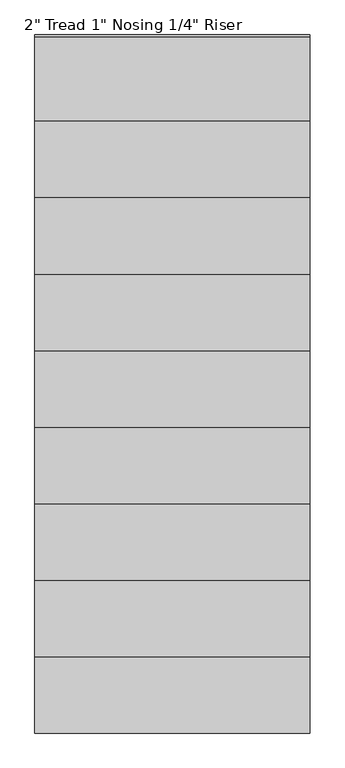
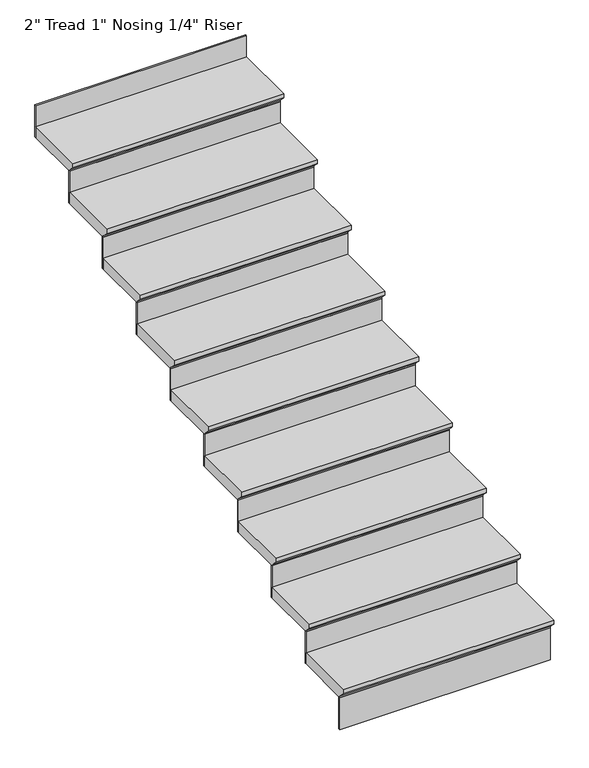
"""IFC4 building model written with IfcOpenShell, lengths in millimetres: stair flight geometry."""

from ifc_helpers import new_model, si_unit, frame, origin, place, context, project, spatial, polyline, outline, extrude, source, transform, mapped, element, save


def stair_flight_ef5934bc(model_context):
    return source(origin(), model_context, "Body", "SweptSolid", [
        extrude(outline(polyline([(-6527.0593836, 7970.3107431), (-6247.6593836, 7970.3107431), (-6247.6593836, 7919.5107431), (-6501.6593836, 7919.5107431), (-6501.6593836, 7925.8607431), (-6527.0593836, 7951.2607431), (-6527.0593836, 7970.3107431)])), frame((-5280.3137331, 0.0, 0.0), z_axis=(1.0, 0.0, 0.0), x_axis=(0.0, 1.0, 0.0)), (0.0, 0.0, 1.0), 914.4),
        extrude(outline(polyline([(-4365.9137331, -6495.3093836), (-4365.9137331, -6501.6593836), (-5280.3137331, -6501.6593836), (-5280.3137331, -6495.3093836), (-4365.9137331, -6495.3093836)])), frame((0.0, 0.0, 7771.6618174), z_axis=(0.0, 0.0, 1.0), x_axis=(1.0, 0.0, 0.0)), (0.0, 0.0, 1.0), 147.8489257),
        extrude(outline(polyline([(-4365.9137331, -6241.3093836), (-4365.9137331, -6247.6593836), (-5280.3137331, -6247.6593836), (-5280.3137331, -6241.3093836), (-4365.9137331, -6241.3093836)])), frame((0.0, 0.0, 7919.5107431), z_axis=(0.0, 0.0, 1.0), x_axis=(1.0, 0.0, 0.0)), (0.0, 0.0, 1.0), 147.8489257),
        extrude(outline(polyline([(-6273.0593836, 8118.1596688), (-5993.6593836, 8118.1596688), (-5993.6593836, 8067.3596688), (-6247.6593836, 8067.3596688), (-6247.6593836, 8073.7096688), (-6273.0593836, 8099.1096688), (-6273.0593836, 8118.1596688)])), frame((-5280.3137331, 0.0, 0.0), z_axis=(1.0, 0.0, 0.0), x_axis=(0.0, 1.0, 0.0)), (0.0, 0.0, 1.0), 914.4),
        extrude(outline(polyline([(-4365.9137331, -5987.3093836), (-4365.9137331, -5993.6593836), (-5280.3137331, -5993.6593836), (-5280.3137331, -5987.3093836), (-4365.9137331, -5987.3093836)])), frame((0.0, 0.0, 8067.3596688), z_axis=(0.0, 0.0, 1.0), x_axis=(1.0, 0.0, 0.0)), (0.0, 0.0, 1.0), 147.8489257),
        extrude(outline(polyline([(-6019.0593836, 8266.0085944), (-5739.6593836, 8266.0085944), (-5739.6593836, 8215.2085944), (-5993.6593836, 8215.2085944), (-5993.6593836, 8221.5585944), (-6019.0593836, 8246.9585944), (-6019.0593836, 8266.0085944)])), frame((-5280.3137331, 0.0, 0.0), z_axis=(1.0, 0.0, 0.0), x_axis=(0.0, 1.0, 0.0)), (0.0, 0.0, 1.0), 914.4),
        extrude(outline(polyline([(-4365.9137331, -5733.3093836), (-4365.9137331, -5739.6593836), (-5280.3137331, -5739.6593836), (-5280.3137331, -5733.3093836), (-4365.9137331, -5733.3093836)])), frame((0.0, 0.0, 8215.2085944), z_axis=(0.0, 0.0, 1.0), x_axis=(1.0, 0.0, 0.0)), (0.0, 0.0, 1.0), 147.8489257),
        extrude(outline(polyline([(-5765.0593836, 8413.8575201), (-5485.6593836, 8413.8575201), (-5485.6593836, 8363.0575201), (-5739.6593836, 8363.0575201), (-5739.6593836, 8369.4075201), (-5765.0593836, 8394.8075201), (-5765.0593836, 8413.8575201)])), frame((-5280.3137331, 0.0, 0.0), z_axis=(1.0, 0.0, 0.0), x_axis=(0.0, 1.0, 0.0)), (0.0, 0.0, 1.0), 914.4),
        extrude(outline(polyline([(-4365.9137331, -5479.3093836), (-4365.9137331, -5485.6593836), (-5280.3137331, -5485.6593836), (-5280.3137331, -5479.3093836), (-4365.9137331, -5479.3093836)])), frame((0.0, 0.0, 8363.0575201), z_axis=(0.0, 0.0, 1.0), x_axis=(1.0, 0.0, 0.0)), (0.0, 0.0, 1.0), 147.8489257),
        extrude(outline(polyline([(-5511.0593836, 8561.7064458), (-5231.6593836, 8561.7064458), (-5231.6593836, 8510.9064458), (-5485.6593836, 8510.9064458), (-5485.6593836, 8517.2564458), (-5511.0593836, 8542.6564458), (-5511.0593836, 8561.7064458)])), frame((-5280.3137331, 0.0, 0.0), z_axis=(1.0, 0.0, 0.0), x_axis=(0.0, 1.0, 0.0)), (0.0, 0.0, 1.0), 914.4),
        extrude(outline(polyline([(-4365.9137331, -5225.3093836), (-4365.9137331, -5231.6593836), (-5280.3137331, -5231.6593836), (-5280.3137331, -5225.3093836), (-4365.9137331, -5225.3093836)])), frame((0.0, 0.0, 8510.9064458), z_axis=(0.0, 0.0, 1.0), x_axis=(1.0, 0.0, 0.0)), (0.0, 0.0, 1.0), 147.8489257),
        extrude(outline(polyline([(-5257.0593836, 8709.5553715), (-4977.6593836, 8709.5553715), (-4977.6593836, 8658.7553715), (-5231.6593836, 8658.7553715), (-5231.6593836, 8665.1053715), (-5257.0593836, 8690.5053715), (-5257.0593836, 8709.5553715)])), frame((-5280.3137331, 0.0, 0.0), z_axis=(1.0, 0.0, 0.0), x_axis=(0.0, 1.0, 0.0)), (0.0, 0.0, 1.0), 914.4),
        extrude(outline(polyline([(-4365.9137331, -4971.3093836), (-4365.9137331, -4977.6593836), (-5280.3137331, -4977.6593836), (-5280.3137331, -4971.3093836), (-4365.9137331, -4971.3093836)])), frame((0.0, 0.0, 8658.7553715), z_axis=(0.0, 0.0, 1.0), x_axis=(1.0, 0.0, 0.0)), (0.0, 0.0, 1.0), 147.8489257),
        extrude(outline(polyline([(-5003.0593836, 8857.4042972), (-4723.6593836, 8857.4042972), (-4723.6593836, 8806.6042972), (-4977.6593836, 8806.6042972), (-4977.6593836, 8812.9542972), (-5003.0593836, 8838.3542972), (-5003.0593836, 8857.4042972)])), frame((-5280.3137331, 0.0, 0.0), z_axis=(1.0, 0.0, 0.0), x_axis=(0.0, 1.0, 0.0)), (0.0, 0.0, 1.0), 914.4),
        extrude(outline(polyline([(-4365.9137331, -4717.3093836), (-4365.9137331, -4723.6593836), (-5280.3137331, -4723.6593836), (-5280.3137331, -4717.3093836), (-4365.9137331, -4717.3093836)])), frame((0.0, 0.0, 8806.6042972), z_axis=(0.0, 0.0, 1.0), x_axis=(1.0, 0.0, 0.0)), (0.0, 0.0, 1.0), 147.8489257),
        extrude(outline(polyline([(-4749.0593836, 9005.2532229), (-4469.6593836, 9005.2532229), (-4469.6593836, 8954.4532229), (-4723.6593836, 8954.4532229), (-4723.6593836, 8960.8032229), (-4749.0593836, 8986.2032229), (-4749.0593836, 9005.2532229)])), frame((-5280.3137331, 0.0, 0.0), z_axis=(1.0, 0.0, 0.0), x_axis=(0.0, 1.0, 0.0)), (0.0, 0.0, 1.0), 914.4),
        extrude(outline(polyline([(-4365.9137331, -4463.3093836), (-4365.9137331, -4469.6593836), (-5280.3137331, -4469.6593836), (-5280.3137331, -4463.3093836), (-4365.9137331, -4463.3093836)])), frame((0.0, 0.0, 8954.4532229), z_axis=(0.0, 0.0, 1.0), x_axis=(1.0, 0.0, 0.0)), (0.0, 0.0, 1.0), 147.8489257),
        extrude(outline(polyline([(-4365.9137331, -4209.3093836), (-4365.9137331, -4215.6593836), (-5280.3137331, -4215.6593836), (-5280.3137331, -4209.3093836), (-4365.9137331, -4209.3093836)])), frame((0.0, 0.0, 9102.3021486), z_axis=(0.0, 0.0, 1.0), x_axis=(1.0, 0.0, 0.0)), (0.0, 0.0, 1.0), 147.8489257),
        extrude(outline(polyline([(-4495.0593836, 9153.1021486), (-4215.6593836, 9153.1021486), (-4215.6593836, 9102.3021486), (-4469.6593836, 9102.3021486), (-4469.6593836, 9108.6521486), (-4495.0593836, 9134.0521486), (-4495.0593836, 9153.1021486)])), frame((-5280.3137331, 0.0, 0.0), z_axis=(1.0, 0.0, 0.0), x_axis=(0.0, 1.0, 0.0)), (0.0, 0.0, 1.0), 914.4),
    ])


if __name__ == "__main__":
    model = new_model("IFC4")
    model_context = context("Model", 3, world=origin())
    ifc_project = project(units=[si_unit("LENGTHUNIT", "METRE", prefix="MILLI")], contexts=[model_context])
    site = spatial("IfcSite", under=ifc_project)
    building = spatial("IfcBuilding", under=site)
    placement = place(None, origin())
    stair_flight_shape = stair_flight_ef5934bc(model_context)
    element("IfcStairFlight", 1, ObjectType="2\" Tread 1\" Nosing 1/4\" Riser", at=placement, inside=building, context=model_context, shape_type="MappedRepresentation", body=[
        mapped(stair_flight_shape, transform((0.0, 0.0, 0.0), x_axis=(1.0, 0.0, 0.0), y_axis=(0.0, 1.0, 0.0), z_axis=(0.0, 0.0, 1.0))),
    ])
    save(model, "model.ifc")
